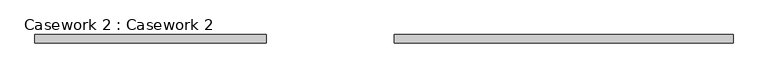
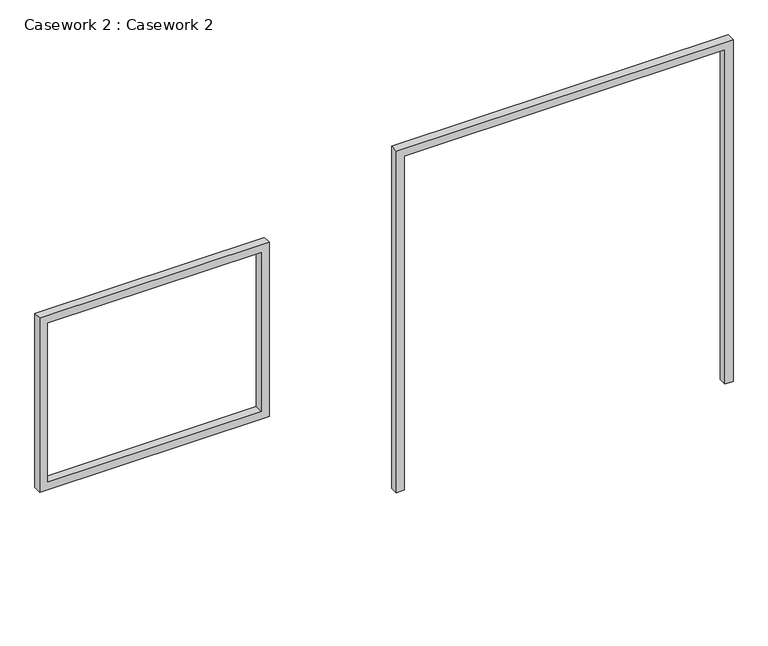
"""IFC4 building model written with IfcOpenShell, lengths in millimetres: furniture geometry, Casework 2 : Casework 2."""

from ifc_helpers import new_model, si_unit, frame, origin, place, context, project, spatial, polyline, outline, extrude, source, transform, mapped, element, save


def casework_2_casework_2_327cef27(model_context):
    return source(origin(), model_context, "Body", "SweptSolid", [
        extrude(outline(polyline([(2546.35, -10737.8417413), (2546.35, -12172.9417413), (1393.8676291, -12172.9417413), (1393.8676291, -10737.8417413), (2546.35, -10737.8417413)]), holes=[polyline([(2495.55, -10788.6417413), (1444.6676291, -10788.6417413), (1444.6676291, -12122.1417413), (2495.55, -12122.1417413), (2495.55, -10788.6417413)])]), frame((0.0, 2409.1965218, 0.0), z_axis=(0.0, 1.0, 0.0), x_axis=(0.0, 0.0, 1.0)), (0.0, 0.0, 1.0), 50.8),
        extrude(outline(polyline([(2819.4, -9892.2917413), (2819.4, -7888.8667413), (609.6, -7888.8667413), (609.6, -7838.0667413), (2870.2, -7838.0667413), (2870.2, -9943.0917413), (609.6, -9943.0917413), (609.6, -9892.2917413), (2819.4, -9892.2917413)])), frame((0.0, 2409.1965218, 0.0), z_axis=(0.0, 1.0, 0.0), x_axis=(0.0, 0.0, 1.0)), (0.0, 0.0, 1.0), 50.8),
    ])


if __name__ == "__main__":
    model = new_model("IFC4")
    model_context = context("Model", 3, world=origin())
    ifc_project = project(units=[si_unit("LENGTHUNIT", "METRE", prefix="MILLI")], contexts=[model_context])
    site = spatial("IfcSite", under=ifc_project)
    building = spatial("IfcBuilding", under=site)
    placement = place(None, origin())
    casework_2_casework_2_shape = casework_2_casework_2_327cef27(model_context)
    element("IfcFurniture", 1, ObjectType="Casework 2 : Casework 2", at=placement, inside=building, context=model_context, shape_type="MappedRepresentation", body=[
        mapped(casework_2_casework_2_shape, transform((0.0, 0.0, 0.0), x_axis=(1.0, 0.0, 0.0), y_axis=(0.0, 1.0, 0.0), z_axis=(0.0, 0.0, 1.0))),
    ])
    save(model, "model.ifc")

# Revit data of these elements
# Element 1 (IfcFurniture, "Casework 2 : Casework 2")
#   Materials on its faces: "Wood Planks"
# Materials
#   "Wood Planks": class "Wood", colour RGB 193 160 115, transparency 0, Description = "Physical material.", Cost = 0
